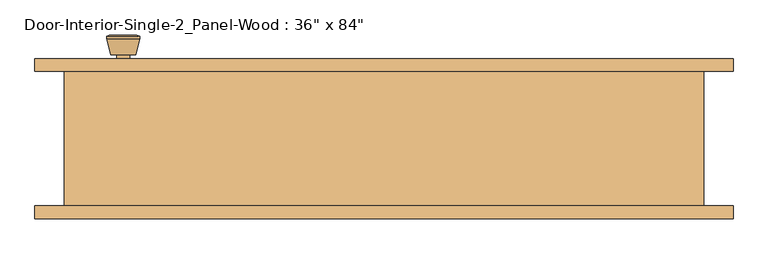
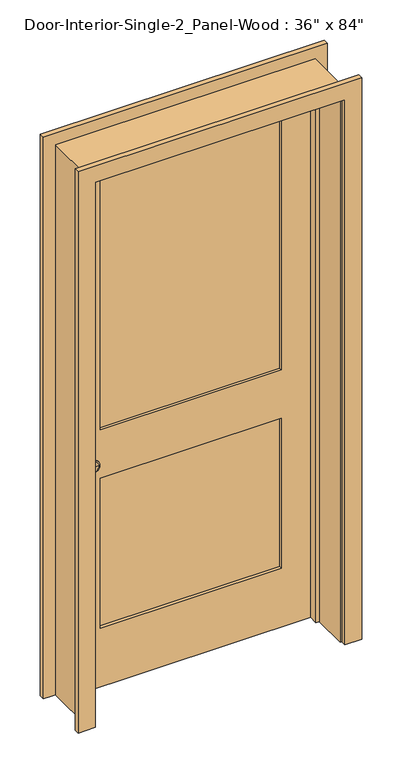
"""IFC4 building model written with IfcOpenShell, lengths in millimetres: door geometry."""

from ifc_helpers import new_model, si_unit, point, frame, frame_2d, origin, place, context, project, spatial, polyline, circle_curve, trimmed, segment, composite_curve, outline, extrude, faceted_brep, source, transform, mapped, element, save
from ifc_brep_helpers import plane_surface, cylinder_surface, revolved_surface, advanced_brep


def door_6f959a6d(model_context):
    return source(origin(), model_context, "Body", "SolidModel", [
        advanced_brep(
        [(-393.7, 57.5, 914.4), (-383.7, 57.5, 914.4), (-403.7, 57.5, 914.4), (-373.2241324, 8.5, 914.4), (-393.7, 8.5, 914.4), (-414.1758676, 8.5, 914.4), (-368.7, 10.3278681, 914.4), (-418.7, 10.3278681, 914.4), (-368.7, 13.7915463, 914.4), (-418.7, 13.7915463, 914.4), (-375.063764, 38.5, 914.4), (-412.336236, 38.5, 914.4), (-383.7, 38.5, 914.4), (-403.7, 38.5, 914.4)],
        [
            (0, 1),
            (1, 2, circle_curve(frame((-393.7, 57.5, 914.4), z_axis=(0.0, 1.0, 0.0), x_axis=(-1.0, 0.0, 0.0)), 10.0)),
            (2, 0),
            (2, 1, circle_curve(frame((-393.7, 57.5, 914.4), z_axis=(0.0, 1.0, 0.0), x_axis=(-1.0, 0.0, 0.0)), 10.0)),
            (3, 4),
            (4, 5),
            (5, 3, circle_curve(frame((-393.7, 8.5, 914.4), z_axis=(0.0, -1.0, 0.0), x_axis=(-1.0, 0.0, 0.0)), 20.4758676)),
            (3, 5, circle_curve(frame((-393.7, 8.5, 914.4), z_axis=(0.0, -1.0, 0.0), x_axis=(-1.0, 0.0, 0.0)), 20.4758676)),
            (6, 3),
            (5, 7),
            (7, 6, circle_curve(frame((-393.7, 10.3278681, 914.4), z_axis=(0.0, -1.0, 0.0), x_axis=(-1.0, 0.0, 0.0)), 25.0)),
            (6, 7, circle_curve(frame((-393.7, 10.3278681, 914.4), z_axis=(0.0, -1.0, 0.0), x_axis=(-1.0, 0.0, 0.0)), 25.0)),
            (8, 6),
            (7, 9),
            (9, 8, circle_curve(frame((-393.7, 13.7915463, 914.4), z_axis=(0.0, -1.0, 0.0), x_axis=(-1.0, 0.0, 0.0)), 25.0)),
            (8, 9, circle_curve(frame((-393.7, 13.7915463, 914.4), z_axis=(0.0, -1.0, 0.0), x_axis=(-1.0, 0.0, 0.0)), 25.0)),
            (10, 8),
            (9, 11),
            (11, 10, circle_curve(frame((-393.7, 38.5, 914.4), z_axis=(0.0, -1.0, 0.0), x_axis=(-1.0, 0.0, 0.0)), 18.636236)),
            (10, 11, circle_curve(frame((-393.7, 38.5, 914.4), z_axis=(0.0, -1.0, 0.0), x_axis=(-1.0, 0.0, 0.0)), 18.636236)),
            (12, 10),
            (11, 13),
            (13, 12, circle_curve(frame((-393.7, 38.5, 914.4), z_axis=(0.0, -1.0, 0.0), x_axis=(-1.0, 0.0, 0.0)), 10.0)),
            (12, 13, circle_curve(frame((-393.7, 38.5, 914.4), z_axis=(0.0, -1.0, 0.0), x_axis=(-1.0, 0.0, 0.0)), 10.0)),
            (1, 12),
            (13, 2),
        ],
        [
            plane_surface(frame((-393.7, 57.5, 914.4), z_axis=(0.0, 1.0, 0.0), x_axis=(-1.0, 0.0, 0.0))),
            plane_surface(frame((-393.7, 8.5, 914.4), z_axis=(0.0, -1.0, 0.0), x_axis=(-1.0, 0.0, 0.0))),
            revolved_surface(polyline([(-414.1758676, 8.5, 914.4), (-418.7, 10.3278681, 914.4)]), (-393.7, 57.5, 914.4), (0.0, 1.0, 0.0)),
            cylinder_surface(frame((-393.7, 57.5, 914.4), z_axis=(0.0, 1.0, 0.0), x_axis=(-1.0, 0.0, 0.0)), 25.0),
            revolved_surface(polyline([(-418.7, 13.7915463, 914.4), (-412.336236, 38.5, 914.4)]), (-393.7, 57.5, 914.4), (0.0, 1.0, 0.0)),
            plane_surface(frame((-393.7, 38.5, 914.4), z_axis=(0.0, 1.0, 0.0), x_axis=(-1.0, 0.0, 0.0))),
            cylinder_surface(frame((-393.7, 57.5, 914.4), z_axis=(0.0, 1.0, 0.0), x_axis=(-1.0, 0.0, 0.0)), 10.0),
        ],
        [
            (0, [[1, 2, 3]]),
            (0, [[-3, 4, -1]]),
            (1, [[5, 6, 7]]),
            (1, [[-6, -5, 8]]),
            (2, [[9, -7, 10, 11]]),
            (2, [[-10, -8, -9, 12]]),
            (3, [[13, -11, 14, 15]]),
            (3, [[-14, -12, -13, 16]]),
            (4, [[17, -15, 18, 19]]),
            (4, [[-18, -16, -17, 20]]),
            (5, [[21, -19, 22, 23]]),
            (5, [[-22, -20, -21, 24]]),
            (6, [[25, -23, 26, -2]]),
            (6, [[-26, -24, -25, -4]]),
        ],
    ),
        extrude(outline(composite_curve([segment(trimmed(circle_curve(frame_2d((914.4, -393.7)), 30.0), [point((914.4, -423.7))], [point((914.4, -363.7))], False, "CARTESIAN"), True, "CONTINUOUS"), segment(trimmed(circle_curve(frame_2d((914.4, -393.7)), 30.0), [point((914.4, -363.7))], [point((914.4, -423.7))], False, "CARTESIAN"), True, "CONTINUOUS")], self_intersect=False)), frame((0.0, 57.5, 0.0), z_axis=(0.0, 1.0, 0.0), x_axis=(0.0, 0.0, 1.0)), (0.0, 0.0, 1.0), 6.0),
        advanced_brep(
        [(-393.7, 104.425, 914.4), (-403.7, 104.425, 914.4), (-383.7, 104.425, 914.4), (-373.2241324, 153.425, 914.4), (-414.1758676, 153.425, 914.4), (-393.7, 153.425, 914.4), (-368.7, 151.5971319, 914.4), (-418.7, 151.5971319, 914.4), (-368.7, 148.1334537, 914.4), (-418.7, 148.1334537, 914.4), (-375.063764, 123.425, 914.4), (-412.336236, 123.425, 914.4), (-383.7, 123.425, 914.4), (-403.7, 123.425, 914.4)],
        [
            (0, 1),
            (1, 2, circle_curve(frame((-393.7, 104.425, 914.4), z_axis=(0.0, -1.0, 0.0), x_axis=(-1.0, 0.0, 0.0)), 10.0)),
            (2, 0),
            (2, 1, circle_curve(frame((-393.7, 104.425, 914.4), z_axis=(0.0, -1.0, 0.0), x_axis=(-1.0, 0.0, 0.0)), 10.0)),
            (3, 4, circle_curve(frame((-393.7, 153.425, 914.4), z_axis=(0.0, 1.0, 0.0), x_axis=(-1.0, 0.0, 0.0)), 20.4758676)),
            (4, 5),
            (5, 3),
            (4, 3, circle_curve(frame((-393.7, 153.425, 914.4), z_axis=(0.0, 1.0, 0.0), x_axis=(-1.0, 0.0, 0.0)), 20.4758676)),
            (6, 7, circle_curve(frame((-393.7, 151.5971319, 914.4), z_axis=(0.0, 1.0, 0.0), x_axis=(-1.0, 0.0, 0.0)), 25.0)),
            (7, 4),
            (3, 6),
            (7, 6, circle_curve(frame((-393.7, 151.5971319, 914.4), z_axis=(0.0, 1.0, 0.0), x_axis=(-1.0, 0.0, 0.0)), 25.0)),
            (8, 9, circle_curve(frame((-393.7, 148.1334537, 914.4), z_axis=(0.0, 1.0, 0.0), x_axis=(-1.0, 0.0, 0.0)), 25.0)),
            (9, 7),
            (6, 8),
            (9, 8, circle_curve(frame((-393.7, 148.1334537, 914.4), z_axis=(0.0, 1.0, 0.0), x_axis=(-1.0, 0.0, 0.0)), 25.0)),
            (10, 11, circle_curve(frame((-393.7, 123.425, 914.4), z_axis=(0.0, 1.0, 0.0), x_axis=(-1.0, 0.0, 0.0)), 18.636236)),
            (11, 9),
            (8, 10),
            (11, 10, circle_curve(frame((-393.7, 123.425, 914.4), z_axis=(0.0, 1.0, 0.0), x_axis=(-1.0, 0.0, 0.0)), 18.636236)),
            (12, 13, circle_curve(frame((-393.7, 123.425, 914.4), z_axis=(0.0, 1.0, 0.0), x_axis=(-1.0, 0.0, 0.0)), 10.0)),
            (13, 11),
            (10, 12),
            (13, 12, circle_curve(frame((-393.7, 123.425, 914.4), z_axis=(0.0, 1.0, 0.0), x_axis=(-1.0, 0.0, 0.0)), 10.0)),
            (1, 13),
            (12, 2),
        ],
        [
            plane_surface(frame((-393.7, 104.425, 914.4), z_axis=(0.0, -1.0, 0.0), x_axis=(-1.0, 0.0, 0.0))),
            plane_surface(frame((-393.7, 153.425, 914.4), z_axis=(0.0, 1.0, 0.0), x_axis=(-1.0, 0.0, 0.0))),
            revolved_surface(polyline([(-414.1758676, 153.425, 914.4), (-418.7, 151.5971319, 914.4)]), (-393.7, 104.425, 914.4), (0.0, -1.0, 0.0)),
            cylinder_surface(frame((-393.7, 104.425, 914.4), z_axis=(0.0, -1.0, 0.0), x_axis=(-1.0, 0.0, 0.0)), 25.0),
            revolved_surface(polyline([(-418.7, 148.1334537, 914.4), (-412.336236, 123.425, 914.4)]), (-393.7, 104.425, 914.4), (0.0, -1.0, 0.0)),
            plane_surface(frame((-393.7, 123.425, 914.4), z_axis=(0.0, -1.0, 0.0), x_axis=(-1.0, 0.0, 0.0))),
            cylinder_surface(frame((-393.7, 104.425, 914.4), z_axis=(0.0, -1.0, 0.0), x_axis=(-1.0, 0.0, 0.0)), 10.0),
        ],
        [
            (0, [[1, 2, 3]]),
            (0, [[-3, 4, -1]]),
            (1, [[5, 6, 7]]),
            (1, [[8, -7, -6]]),
            (2, [[9, 10, -5, 11]]),
            (2, [[12, -11, -8, -10]]),
            (3, [[13, 14, -9, 15]]),
            (3, [[16, -15, -12, -14]]),
            (4, [[17, 18, -13, 19]]),
            (4, [[20, -19, -16, -18]]),
            (5, [[21, 22, -17, 23]]),
            (5, [[24, -23, -20, -22]]),
            (6, [[-2, 25, -21, 26]]),
            (6, [[-4, -26, -24, -25]]),
        ],
    ),
        extrude(outline(composite_curve([segment(trimmed(circle_curve(frame_2d((914.4, -393.7)), 30.0), [point((914.4, -423.7))], [point((914.4, -363.7))], False, "CARTESIAN"), True, "CONTINUOUS"), segment(trimmed(circle_curve(frame_2d((914.4, -393.7)), 30.0), [point((914.4, -363.7))], [point((914.4, -423.7))], False, "CARTESIAN"), True, "CONTINUOUS")], self_intersect=False)), frame((0.0, 98.425, 0.0), z_axis=(0.0, 1.0, 0.0), x_axis=(0.0, 0.0, 1.0)), (0.0, 0.0, 1.0), 6.0),
        extrude(outline(polyline([(336.55, 75.1416667), (-336.55, 75.1416667), (-336.55, 86.7833333), (336.55, 86.7833333), (336.55, 75.1416667)])), frame((0.0, 0.0, 1009.65), z_axis=(0.0, 0.0, 1.0), x_axis=(1.0, 0.0, 0.0)), (0.0, 0.0, 1.0), 1004.8875),
        extrude(outline(polyline([(336.55, 75.1416667), (-336.55, 75.1416667), (-336.55, 86.7833333), (336.55, 86.7833333), (336.55, 75.1416667)])), frame((0.0, 0.0, 231.775), z_axis=(0.0, 0.0, 1.0), x_axis=(1.0, 0.0, 0.0)), (0.0, 0.0, 1.0), 587.375),
        extrude(outline(polyline([(2133.6, -457.2), (0.0, -457.2), (0.0, 457.2), (2133.6, 457.2), (2133.6, -457.2)]), holes=[polyline([(2014.5375, -336.55), (2014.5375, 336.55), (1009.65, 336.55), (1009.65, -336.55), (2014.5375, -336.55)]), polyline([(819.15, -336.55), (819.15, 336.55), (231.775, 336.55), (231.775, -336.55), (819.15, -336.55)])]), frame((0.0, 63.5, 0.0), z_axis=(0.0, 1.0, 0.0), x_axis=(0.0, 0.0, 1.0)), (0.0, 0.0, 1.0), 34.925),
        faceted_brep([(482.6, 98.425, 0.0), (482.6, -104.775, 0.0), (457.2, -104.775, 0.0), (457.2, 28.575, 0.0), (444.5, 28.575, 0.0), (444.5, 63.5, 0.0), (457.2, 63.5, 0.0), (457.2, 98.425, 0.0), (482.6, 98.425, 2159.0), (482.6, -104.775, 2159.0), (-482.6, -104.775, 2159.0), (-482.6, -104.775, 0.0), (-457.2, -104.775, 0.0), (-457.2, -104.775, 2133.6), (457.2, -104.775, 2133.6), (457.2, 28.575, 2133.6), (-457.2, 28.575, 2133.6), (-457.2, 28.575, 0.0), (-444.5, 28.575, 0.0), (-444.5, 28.575, 2120.9), (444.5, 28.575, 2120.9), (444.5, 63.5, 2120.9), (-444.5, 63.5, 2120.9), (-444.5, 63.5, 0.0), (-457.2, 63.5, 0.0), (-457.2, 63.5, 2133.6), (457.2, 63.5, 2133.6), (457.2, 98.425, 2133.6), (-457.2, 98.425, 2133.6), (-457.2, 98.425, 0.0), (-482.6, 98.425, 0.0), (-482.6, 98.425, 2159.0)], [[[0, 1, 2, 3, 4, 5, 6, 7]], [[1, 0, 8, 9]], [[2, 1, 9, 10, 11, 12, 13, 14]], [[3, 2, 14, 15]], [[4, 3, 15, 16, 17, 18, 19, 20]], [[5, 4, 20, 21]], [[6, 5, 21, 22, 23, 24, 25, 26]], [[7, 6, 26, 27]], [[0, 7, 27, 28, 29, 30, 31, 8]], [[9, 8, 31, 10]], [[15, 14, 13, 16]], [[21, 20, 19, 22]], [[27, 26, 25, 28]], [[30, 29, 24, 23, 18, 17, 12, 11]], [[10, 31, 30, 11]], [[16, 13, 12, 17]], [[22, 19, 18, 23]], [[28, 25, 24, 29]]]),
        extrude(outline(polyline([(0.0, 463.55), (0.0, 527.05), (2203.45, 527.05), (2203.45, -527.05), (0.0, -527.05), (0.0, -463.55), (2139.95, -463.55), (2139.95, 463.55), (0.0, 463.55)])), frame((0.0, -123.825, 0.0), z_axis=(0.0, 1.0, 0.0), x_axis=(0.0, 0.0, 1.0)), (0.0, 0.0, 1.0), 19.05),
        extrude(outline(polyline([(0.0, 463.55), (0.0, 527.05), (2203.45, 527.05), (2203.45, -527.05), (0.0, -527.05), (0.0, -463.55), (2139.95, -463.55), (2139.95, 463.55), (0.0, 463.55)])), frame((0.0, 98.425, 0.0), z_axis=(0.0, 1.0, 0.0), x_axis=(0.0, 0.0, 1.0)), (0.0, 0.0, 1.0), 19.05),
    ])


if __name__ == "__main__":
    model = new_model("IFC4")
    model_context = context("Model", 3, world=origin())
    ifc_project = project(units=[si_unit("LENGTHUNIT", "METRE", prefix="MILLI")], contexts=[model_context])
    site = spatial("IfcSite", under=ifc_project)
    building = spatial("IfcBuilding", under=site)
    placement = place(None, origin())
    door_shape = door_6f959a6d(model_context)
    element("IfcDoor", 1, ObjectType="Door-Interior-Single-2_Panel-Wood : 36\" x 84\"", at=placement, inside=building, context=model_context, shape_type="MappedRepresentation", body=[
        mapped(door_shape, transform((0.0, 0.0, 0.0), x_axis=(1.0, 0.0, 0.0), y_axis=(0.0, 1.0, 0.0), z_axis=(0.0, 0.0, 1.0))),
    ])
    save(model, "model.ifc")

# Revit data of these elements
# Type "Door-Interior-Single-2_Panel-Wood : 36\" x 84\""
#   Type Mark = "11"
#   Assembly Code = "C1020300"
#   Analytic Construction = "Wooden"
#   Top Rail = 0' - 4 11/16"
#   Thickness = 0' - 1 3/8"
#   Thermal Resistance (R) = 2.5876 (h·ft²·°F)/BTU
#   Swing Angle [instance default] = 90.00°
#   Stiles = 0' - 4 3/4"
#   Rough Width = 3' - 2"
#   Rough Height = 7' - 1"
#   Lock Rail = 0' - 7 1/2"
#   Height = 7' - 0"
#   Width = 3' - 0"
#   Heat Transfer Coefficient (U) = 0.3865 BTU/(h·ft²·°F)
#   Bottom Rail = 0' - 9 1/8"
#   Trim Material = Cherry
#   Panel Material = Cherry
#   Frame Material = Cherry
#   Door Handle Material = Aluminum
#   Visual Light Transmittance = 0
#   Solar Heat Gain Coefficient = 0
#   Wall Closure = (empty or 0)
#   Function = (empty or 0)
# Element 1 (IfcDoor, "Door-Interior-Single-2_Panel-Wood : 36\" x 84\"")
#   Materials on its faces: "Cherry", "Aluminum"
# Materials
#   "Cherry": class "Wood", colour RGB 226 177 128, transparency 0, Description = "Prunus Serotina", Cost = 0
#   "Aluminum": class "Metal", colour RGB 247 247 247, transparency 0, Description = "Aluminum 6061", Cost = 0
